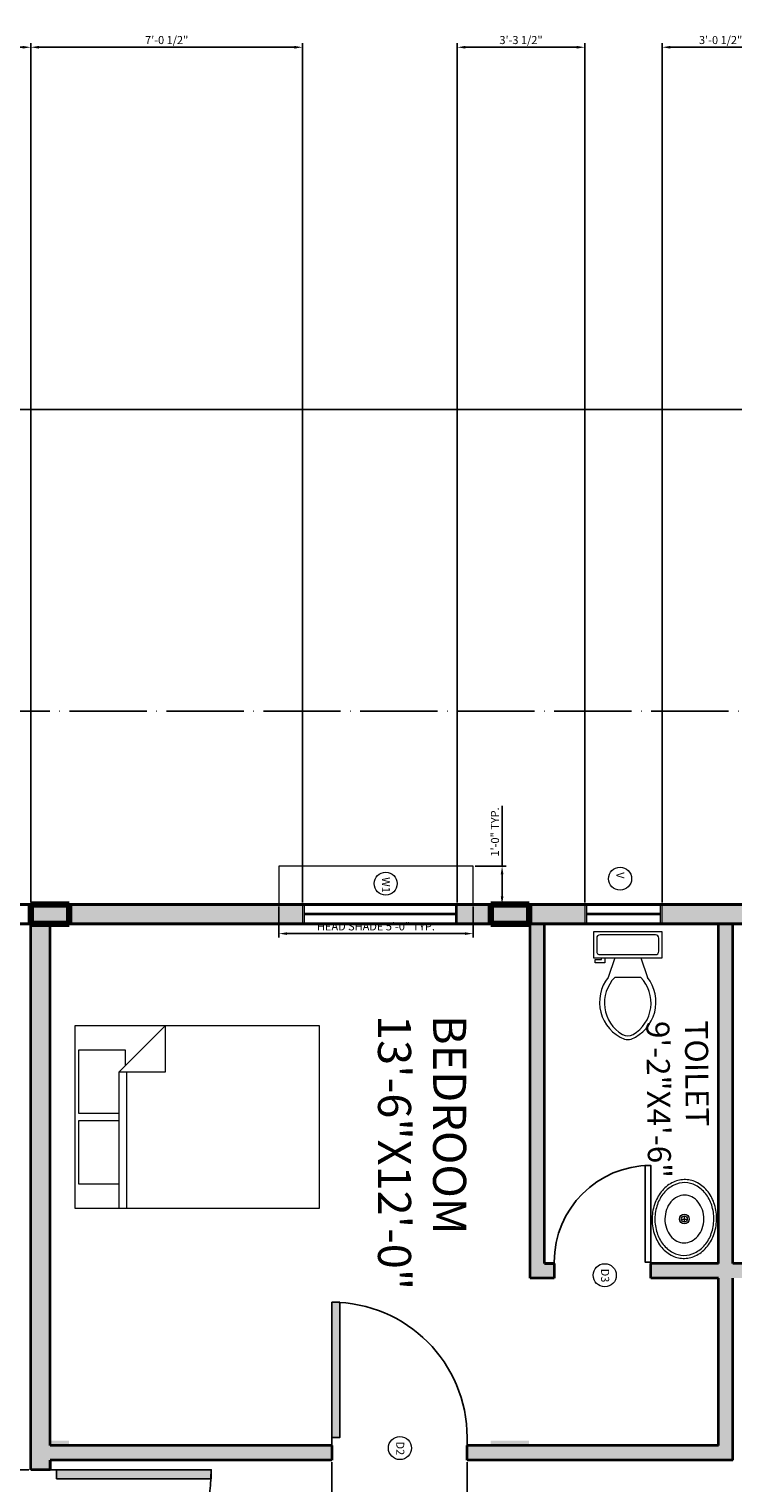
# Model space of a CAD drawing. Units: inches. Extents: x 7028582 to 7030319, y 63109697 to 63111305.
# Tile 17 of 18: x 7029748 to 7029966, y 63110853 to 63111305. Entities that reach past the tile are written whole.
import ezdxf

# ---------------------------------------------------------------- set-up
doc = ezdxf.new("R2010")
doc.units = ezdxf.units.IN
doc.linetypes.add('ACAD_ISO04W100', pattern=[30, 24, -3, 0, -3])
for name, color, linetype, lineweight in [('A-AREA-IDEN', 7, 'Continuous', 18), ('A-DOOR-IDEN', 20, 'Continuous', 13), ('A-FLOR-FIXT', 9, 'Continuous', 18), ('A-GLAZ-IDEN', 20, 'Continuous', 13), ('A-WALL-PATT', 8, 'Continuous', 13), ('C-ANNO-DIMS', 7, 'Continuous', 18), ('C-PROP', 1, 'ACAD_ISO04W100', 25), ('doors', 20, 'Continuous', 25), ('furniture', 9, 'Continuous', 18), ('PILLARS', 220, 'Continuous', 100), ('S-COLS-PATT', 220, 'Continuous', 100), ('walls', 6, 'Continuous', 35), ('WINDOW SHADOW', 9, 'Continuous', 13), ('windows', 5, 'Continuous', 18)]:
    doc.layers.add(name, color=color, linetype=linetype, lineweight=lineweight)
doc.styles.get("Standard").update_dxf_attribs({"font": 'arial.ttf'})
doc.dimstyles.new('ISO-25', dxfattribs={"dimtxt": 2.5, "dimasz": 2.5, "dimexe": 1.25, "dimexo": 0.625, "dimtad": 1, "dimlunit": 4, "dimtxsty": 'Standard', "dimcen": 2.5, "dimadec": 0, "dimazin": 0, "dimtfac": 1, "dimtmove": 0, "dimatfit": 3, "dimfxl": 1, "dimarcsym": 0})

# ---------------------------------------------------------------- blocks, each defined once
blk = doc.blocks.new('*U2')
for p, q in [((0, 0), (0, -5)), ((30, 0), (30, -5))]:
    blk.add_line(p, q)
blk.add_lwpolyline([(0, 0), (0, 30), (1.75, 30), (1.75, 0)], close=True)
blk.add_arc((0, 0), 30, 0, 90)
blk = doc.blocks.new('Toilet - top')
for p, q in [((9.5, -6), (9.5, -2)), ((-10, -8.5), (-8, -8.5)), ((-10, -9.5), (-10, -8.5)), ((-8, -8.5), (-8, -8)), ((-7, -8), (-7, -9.5)), ((-4, -8), (-6, -14)), ((4, -8), (6, -14)), ((-7, -9.5), (-10, -9.5)), ((4, -14), (-4, -14))]:
    blk.add_line(p, q)
blk.add_lwpolyline([(10.5, -8), (10.5, 0), (-10.5, 0), (-10.5, -8)], close=True)
for points in [[(-9.5, -2), (-9.5, -6)], [(8.5, -1), (-8.5, -1)], [(-8.5, -7), (8.5, -7)]]:
    blk.add_lwpolyline(points)
for centre, radius, start, end in [((-8.62, -1.88), 0.884, 81.8699, 188.1301), ((8.62, -1.88), 0.884, 351.8699, 98.1301), ((-8.62, -6.12), 0.884, 171.8699, 278.1301), ((8.62, -6.12), 0.884, 261.8699, 8.1301), ((3.52, -21.58), 12.17, 141.4691, 247.9714), ((4.2, -21.82), 11.33, 136.3677, 238.9468), ((-3.52, -21.58), 12.17, 292.0284, 38.5307), ((-4.2, -21.82), 11.33, 301.053, 43.6321), ((0, -27.88), 4, 245.7318, 294.2682), ((0, -29), 4, 254.8605, 285.1395)]:
    blk.add_arc(centre, radius, start, end)
blk = doc.blocks.new('Sink - Oval top')
for p, q in [((-1, 0), (1, 0)), ((0, 1), (0, -1))]:
    blk.add_line(p, q)
for points in [[(-12.23, 0.39, 0.117634), (-11.46, -3.36, 0.104469), (-8.88, -6.8, 0.090016), (-5.08, -9.07, 0.08192), (-0.32, -10.02, 0.08192), (4.49, -9.38, 0.090016), (8.42, -7.36, 0.104469), (11.22, -4.09, 0.117634), (12.23, -0.39, 0.117634), (11.46, 3.36, 0.104469), (8.88, 6.8, 0.090016), (5.08, 9.07, 0.08192), (0.32, 10.02, 0.08192), (-4.49, 9.38, 0.090016), (-8.42, 7.36, 0.104469), (-11.22, 4.09, 0.117634)], [(-11.29, 0.16, 0.118622), (-10.52, -3.25, 0.104678), (-8.07, -6.36, 0.089562), (-4.54, -8.37, 0.081185), (-0.13, -9.15, 0.081185), (4.3, -8.49, 0.089562), (7.89, -6.58, 0.104678), (10.42, -3.55, 0.118622), (11.29, -0.16, 0.118622), (10.52, 3.25, 0.104678), (8.07, 6.36, 0.089562), (4.54, 8.37, 0.081185), (0.13, 9.15, 0.081185), (-4.3, 8.49, 0.089562), (-7.89, 6.58, 0.104678), (-10.42, 3.55, 0.118622)], [(-7.42, 0.08, 0.118283), (-6.91, -2.17, 0.104607), (-5.29, -4.21, 0.089718), (-2.97, -5.53, 0.081436), (-0.07, -6.04, 0.081436), (2.84, -5.59, 0.089718), (5.2, -4.33, 0.104607), (6.86, -2.32, 0.118283), (7.42, -0.08, 0.118283), (6.91, 2.17, 0.104607), (5.29, 4.21, 0.089718), (2.97, 5.53, 0.081436), (0.07, 6.04, 0.081436), (-2.84, 5.59, 0.089718), (-5.2, 4.33, 0.104607), (-6.86, 2.32, 0.118283)]]:
    blk.add_lwpolyline(points, format="xyb", close=True)
for radius in [1.5, 1]:
    blk.add_circle((0, 0), radius)
blk = doc.blocks.new('Bed - Queen')
for p, q in [((0, -80.00003), (0, 0)), ((0, 0), (59.99999, 0)), ((59.99999, 0), (59.99999, -80.00003)), ((7.99999, -1.2), (28.79998, -1.2)), ((7.99999, -14.4), (7.99999, -1.2)), ((28.79998, -1.2), (28.79998, -14.4)), ((31.19999, -1.2), (51.99999, -1.2)), ((31.19999, -14.4), (31.19999, -1.2)), ((51.99999, -1.2), (51.99999, -16.4)), ((0, -14.4), (44.8, -14.4)), ((44.8, -16.8), (0, -16.8)), ((59.99999, -29.6), (44.8, -14.4)), ((44.8, -14.4), (44.8, -29.6)), ((51.99999, -16.4), (46.79936, -16.4)), ((44.8, -29.6), (59.99999, -29.6)), ((59.99999, -80.00003), (0, -80.00003))]:
    blk.add_line(p, q)
blk = doc.blocks.new('*D11')
at = {"layer": 'C-ANNO-DIMS', "color": 0, "lineweight": -2, "transparency": 16777216}
for p, q in [((7029174.71, 63111093.68), (7029174.71, 63111188.03)), ((7030233.21, 63111186.78), (7029177.21, 63111186.78)), ((7030235.71, 63111093.68), (7030235.71, 63111188.03))]:
    blk.add_line(p, q, dxfattribs=at)
at = {"layer": 'C-ANNO-DIMS', "color": 0, "lineweight": 100, "transparency": 16777216}
for points in [[(7029177.21, 63111187.2), (7029177.21, 63111186.36), (7029174.71, 63111186.78)], [(7030233.21, 63111187.2), (7030233.21, 63111186.36), (7030235.71, 63111186.78)]]:
    blk.add_solid(points, dxfattribs=at)
at = {"layer": 'Defpoints', "color": 0, "lineweight": 100, "transparency": 16777216}
for p in [(7029174.71, 63111186.78), (7029174.71, 63111093.06), (7030235.71, 63111093.06)]:
    blk.add_point(p, dxfattribs=at)
at = {"layer": 'C-ANNO-DIMS', "color": 0, "transparency": 16777216, "insert": (7029705.21, 63111193.53), "char_height": 12, "attachment_point": 5}
blk.add_mtext('88\'-5"', dxfattribs=at)
blk = doc.blocks.new('WIN-SASH-24')
for p, q in [((24.05, 6), (0, 6)), ((0.5, 6), (0.5, 0)), ((23.55, 0), (23.55, 6)), ((0, 0), (24.05, 0)), ((23.55, 3.2), (0.5, 3.2)), ((23.55, 2.8), (0.5, 2.8))]:
    blk.add_line(p, q)
blk = doc.blocks.new('WIN-SASH-48')
for p, q in [((48.05, 6), (0, 6)), ((0.5, 6), (0.5, 0)), ((47.55, 0), (47.55, 6)), ((47.55, 3.2), (0.5, 3.2)), ((47.55, 2.8), (0.5, 2.8)), ((0, 0), (48.05, 0))]:
    blk.add_line(p, q)
blk = doc.blocks.new('WINDOW-SHADE-HEAD-60')
for p, q in [((60.25, 11.9), (0, 11.9)), ((0, 11.9), (0, 0)), ((60.25, 0), (60.25, 11.9))]:
    blk.add_line(p, q)
blk = doc.blocks.new('TAG-D2-MT-R')
blk.add_circle((3.58, 3.58), 3.58)
at = {"insert": (4.93, 5.6), "char_height": 2.5, "attachment_point": 1, "rotation": 270}
blk.add_mtext_dynamic_manual_height_columns('D2', width=2.5021, gutter_width=12.5, heights=[0], dxfattribs=at)
blk = doc.blocks.new('TAG-D3-MT-R')
blk.add_circle((3.58, 3.58), 3.58)
at = {"insert": (4.93, 5.6), "char_height": 2.5, "attachment_point": 1, "rotation": 270}
blk.add_mtext_dynamic_manual_height_columns('D3', width=2.5021, gutter_width=12.5, heights=[0], dxfattribs=at)
blk = doc.blocks.new('TAG-V-MT-R')
blk.add_circle((3.58, 3.58), 3.58)
at = {"insert": (4.93, 5.6), "char_height": 2.5, "attachment_point": 1, "rotation": 270}
blk.add_mtext_dynamic_manual_height_columns('V', width=2.5021, gutter_width=12.5, heights=[0], dxfattribs=at)
blk = doc.blocks.new('TAG-W1-MT-R')
blk.add_circle((3.58, 3.58), 3.58)
at = {"insert": (4.93, 5.6), "char_height": 2.5, "attachment_point": 1, "rotation": 270}
blk.add_mtext_dynamic_manual_height_columns('W1', width=2.5021, gutter_width=12.5, heights=[0], dxfattribs=at)
blk = doc.blocks.new('*D91')
at = {"layer": 'C-ANNO-DIMS', "color": 0, "lineweight": -2, "transparency": 16777216}
for p, q in [((7029825.25, 63111032.43), (7029825.25, 63111022.77)), ((7029885.5, 63111032.43), (7029885.5, 63111022.77)), ((7029827.75, 63111024.02), (7029883, 63111024.02))]:
    blk.add_line(p, q, dxfattribs=at)
at = {"layer": 'C-ANNO-DIMS', "color": 0, "lineweight": 100, "transparency": 16777216}
for points in [[(7029827.75, 63111024.44), (7029827.75, 63111023.6), (7029825.25, 63111024.02)], [(7029883, 63111024.44), (7029883, 63111023.6), (7029885.5, 63111024.02)]]:
    blk.add_solid(points, dxfattribs=at)
at = {"layer": 'Defpoints', "color": 0, "lineweight": 100, "transparency": 16777216}
for p in [(7029825.25, 63111033.06), (7029885.5, 63111033.06), (7029885.5, 63111024.02)]:
    blk.add_point(p, dxfattribs=at)
at = {"layer": 'C-ANNO-DIMS', "color": 0, "transparency": 16777216, "insert": (7029855.37, 63111025.94), "char_height": 2.5, "attachment_point": 5}
blk.add_mtext('HEAD SHADE 5\'-0" TYP.', dxfattribs=at)
blk = doc.blocks.new('*D92')
at = {"layer": 'C-ANNO-DIMS', "color": 0, "lineweight": -2, "transparency": 16777216}
for p, q in [((7029894.53, 63111044.96), (7029894.53, 63111063.71)), ((7029886.12, 63111044.96), (7029895.78, 63111044.96)), ((7029894.53, 63111035.56), (7029894.53, 63111042.46)), ((7029886.12, 63111033.06), (7029895.78, 63111033.06))]:
    blk.add_line(p, q, dxfattribs=at)
at = {"layer": 'C-ANNO-DIMS', "color": 0, "lineweight": 100, "transparency": 16777216}
for points in [[(7029894.12, 63111042.46), (7029894.95, 63111042.46), (7029894.53, 63111044.96)], [(7029894.12, 63111035.56), (7029894.95, 63111035.56), (7029894.53, 63111033.06)]]:
    blk.add_solid(points, dxfattribs=at)
at = {"layer": 'Defpoints', "color": 0, "lineweight": 100, "transparency": 16777216}
for p in [(7029885.5, 63111044.96), (7029894.53, 63111044.96), (7029885.5, 63111033.06)]:
    blk.add_point(p, dxfattribs=at)
at = {"layer": 'C-ANNO-DIMS', "color": 0, "transparency": 16777216, "insert": (7029892.63, 63111055.58), "char_height": 2.5, "attachment_point": 5, "rotation": 90}
blk.add_mtext('1\'-0" TYP.', dxfattribs=at)
blk = doc.blocks.new('*D102')
at = {"layer": 'C-ANNO-DIMS', "color": 0, "lineweight": -2, "transparency": 16777216}
for p, q in [((7029662.21, 63111033.68), (7029662.21, 63111300.44)), ((7029664.71, 63111299.19), (7029745.71, 63111299.19)), ((7029748.21, 63111033.68), (7029748.21, 63111300.44))]:
    blk.add_line(p, q, dxfattribs=at)
at = {"layer": 'C-ANNO-DIMS', "color": 0, "lineweight": 100, "transparency": 16777216}
for points in [[(7029664.71, 63111299.61), (7029664.71, 63111298.77), (7029662.21, 63111299.19)], [(7029745.71, 63111299.61), (7029745.71, 63111298.77), (7029748.21, 63111299.19)]]:
    blk.add_solid(points, dxfattribs=at)
at = {"layer": 'Defpoints', "color": 0, "lineweight": 100, "transparency": 16777216}
for p in [(7029748.21, 63111299.19), (7029662.21, 63111033.06), (7029748.21, 63111033.06)]:
    blk.add_point(p, dxfattribs=at)
at = {"layer": 'C-ANNO-DIMS', "color": 0, "transparency": 16777216, "insert": (7029705.21, 63111301.07), "char_height": 2.5, "attachment_point": 5}
blk.add_mtext('7\'-2"', dxfattribs=at)
blk = doc.blocks.new('*D104')
at = {"layer": 'C-ANNO-DIMS', "color": 0, "lineweight": -2, "transparency": 16777216}
for p, q in [((7029747.58, 63110857.56), (7028586.23, 63110857.56)), ((7028587.48, 63110812.06), (7028587.48, 63110855.06)), ((7029747.58, 63110809.56), (7028586.23, 63110809.56))]:
    blk.add_line(p, q, dxfattribs=at)
at = {"layer": 'C-ANNO-DIMS', "color": 0, "lineweight": 100, "transparency": 16777216}
for points in [[(7028587.06, 63110855.06), (7028587.89, 63110855.06), (7028587.48, 63110857.56)], [(7028587.06, 63110812.06), (7028587.89, 63110812.06), (7028587.48, 63110809.56)]]:
    blk.add_solid(points, dxfattribs=at)
at = {"layer": 'Defpoints', "color": 0, "lineweight": 100, "transparency": 16777216}
for p in [(7028587.48, 63110857.56), (7029748.21, 63110857.56), (7029748.21, 63110809.56)]:
    blk.add_point(p, dxfattribs=at)
at = {"layer": 'C-ANNO-DIMS', "color": 0, "transparency": 16777216, "insert": (7028585.57, 63110833.56), "char_height": 2.5, "attachment_point": 5, "rotation": 90}
blk.add_mtext('4\'-0"', dxfattribs=at)
blk = doc.blocks.new('*D105')
at = {"layer": 'C-ANNO-DIMS', "color": 0, "lineweight": -2, "transparency": 16777216}
for p, q in [((7029841.68, 63110859.93), (7029841.68, 63109697.14)), ((7029883.68, 63110859.93), (7029883.68, 63109697.14)), ((7029844.18, 63109698.39), (7029881.18, 63109698.39))]:
    blk.add_line(p, q, dxfattribs=at)
at = {"layer": 'C-ANNO-DIMS', "color": 0, "lineweight": 100, "transparency": 16777216}
for points in [[(7029844.18, 63109698.8), (7029844.18, 63109697.97), (7029841.68, 63109698.39)], [(7029881.18, 63109698.8), (7029881.18, 63109697.97), (7029883.68, 63109698.39)]]:
    blk.add_solid(points, dxfattribs=at)
at = {"layer": 'Defpoints', "color": 0, "lineweight": 100, "transparency": 16777216}
for p in [(7029841.68, 63110860.56), (7029883.68, 63110860.56), (7029883.68, 63109698.39)]:
    blk.add_point(p, dxfattribs=at)
at = {"layer": 'C-ANNO-DIMS', "color": 0, "transparency": 16777216, "insert": (7029862.68, 63109700.29), "char_height": 2.5, "attachment_point": 5}
blk.add_mtext('3\'-6"', dxfattribs=at)
blk = doc.blocks.new('*D112')
at = {"layer": 'C-ANNO-DIMS', "color": 0, "lineweight": -2, "transparency": 16777216}
for p, q in [((7029747.58, 63111033.06), (7028586.23, 63111033.06)), ((7028587.48, 63111030.56), (7028587.48, 63110548.06)), ((7029747.58, 63110545.56), (7028586.23, 63110545.56))]:
    blk.add_line(p, q, dxfattribs=at)
at = {"layer": 'C-ANNO-DIMS', "color": 0, "lineweight": 100, "transparency": 16777216}
for points in [[(7028587.06, 63111030.56), (7028587.89, 63111030.56), (7028587.48, 63111033.06)], [(7028587.06, 63110548.06), (7028587.89, 63110548.06), (7028587.48, 63110545.56)]]:
    blk.add_solid(points, dxfattribs=at)
at = {"layer": 'Defpoints', "color": 0, "lineweight": 100, "transparency": 16777216}
for p in [(7029748.21, 63111033.06), (7028587.48, 63110545.56), (7029748.21, 63110545.56)]:
    blk.add_point(p, dxfattribs=at)
at = {"layer": 'C-ANNO-DIMS', "color": 0, "transparency": 16777216, "insert": (7028585.56, 63110789.31), "char_height": 2.5, "attachment_point": 5, "rotation": 90}
blk.add_mtext('40\'-7 1/2"', dxfattribs=at)
blk = doc.blocks.new('*D113')
at = {"layer": 'C-ANNO-DIMS', "color": 0, "lineweight": -2, "transparency": 16777216}
for p, q in [((7029748.21, 63111033.68), (7029748.21, 63111300.44)), ((7029750.71, 63111299.19), (7029830.07, 63111299.19)), ((7029832.57, 63111033.68), (7029832.57, 63111300.44))]:
    blk.add_line(p, q, dxfattribs=at)
at = {"layer": 'C-ANNO-DIMS', "color": 0, "lineweight": 100, "transparency": 16777216}
for points in [[(7029750.71, 63111299.61), (7029750.71, 63111298.77), (7029748.21, 63111299.19)], [(7029830.07, 63111299.61), (7029830.07, 63111298.77), (7029832.57, 63111299.19)]]:
    blk.add_solid(points, dxfattribs=at)
at = {"layer": 'Defpoints', "color": 0, "lineweight": 100, "transparency": 16777216}
for p in [(7029832.57, 63111299.19), (7029748.21, 63111033.06), (7029832.57, 63111033.06)]:
    blk.add_point(p, dxfattribs=at)
at = {"layer": 'C-ANNO-DIMS', "color": 0, "transparency": 16777216, "insert": (7029790.39, 63111301.11), "char_height": 2.5, "attachment_point": 5}
blk.add_mtext('7\'-0 1/2"', dxfattribs=at)
blk = doc.blocks.new('*D114')
at = {"layer": 'C-ANNO-DIMS', "color": 0, "lineweight": -2, "transparency": 16777216}
for p, q in [((7029880.62, 63111033.68), (7029880.62, 63111300.44)), ((7029883.12, 63111299.19), (7029917.71, 63111299.19)), ((7029920.21, 63111033.68), (7029920.21, 63111300.44))]:
    blk.add_line(p, q, dxfattribs=at)
at = {"layer": 'C-ANNO-DIMS', "color": 0, "lineweight": 100, "transparency": 16777216}
for points in [[(7029883.12, 63111299.61), (7029883.12, 63111298.77), (7029880.62, 63111299.19)], [(7029917.71, 63111299.61), (7029917.71, 63111298.77), (7029920.21, 63111299.19)]]:
    blk.add_solid(points, dxfattribs=at)
at = {"layer": 'Defpoints', "color": 0, "lineweight": 100, "transparency": 16777216}
for p in [(7029920.21, 63111299.19), (7029880.62, 63111033.06), (7029920.21, 63111033.06)]:
    blk.add_point(p, dxfattribs=at)
at = {"layer": 'C-ANNO-DIMS', "color": 0, "transparency": 16777216, "insert": (7029900.41, 63111301.11), "char_height": 2.5, "attachment_point": 5}
blk.add_mtext('3\'-3 1/2"', dxfattribs=at)
blk = doc.blocks.new('*D115')
at = {"layer": 'C-ANNO-DIMS', "color": 0, "lineweight": -2, "transparency": 16777216}
for p, q in [((7029944.26, 63111033.68), (7029944.26, 63111300.44)), ((7029946.76, 63111299.19), (7029978.03, 63111299.19)), ((7029980.53, 63111033.68), (7029980.53, 63111300.44))]:
    blk.add_line(p, q, dxfattribs=at)
at = {"layer": 'C-ANNO-DIMS', "color": 0, "lineweight": 100, "transparency": 16777216}
for points in [[(7029946.76, 63111299.61), (7029946.76, 63111298.77), (7029944.26, 63111299.19)], [(7029978.03, 63111299.61), (7029978.03, 63111298.77), (7029980.53, 63111299.19)]]:
    blk.add_solid(points, dxfattribs=at)
at = {"layer": 'Defpoints', "color": 0, "lineweight": 100, "transparency": 16777216}
for p in [(7029980.53, 63111299.19), (7029944.26, 63111033.06), (7029980.53, 63111033.06)]:
    blk.add_point(p, dxfattribs=at)
at = {"layer": 'C-ANNO-DIMS', "color": 0, "transparency": 16777216, "insert": (7029962.39, 63111301.11), "char_height": 2.5, "attachment_point": 5}
blk.add_mtext('3\'-0 1/2"', dxfattribs=at)

msp = doc.modelspace()

# ---------------------------------------------------------------- hatches: boundary and pattern name
at = {"layer": 'A-WALL-PATT'}
h = msp.add_hatch(color=256, dxfattribs=at)
h.dxf.hatch_style = 1
h.paths.add_polyline_path([(7029832.57, 63111033.057), (7029748.205, 63111033.057), (7029748.205, 63111027.057), (7029832.57, 63111027.057)])
h = msp.add_hatch(color=256, dxfattribs=at)
h.dxf.hatch_style = 1
h.paths.add_polyline_path([(7029920.21, 63111033.057), (7029880.618, 63111033.057), (7029880.618, 63111027.057), (7029920.21, 63111027.057)])
h = msp.add_hatch(color=256, dxfattribs=at)
h.dxf.hatch_style = 1
h.paths.add_polyline_path([(7029980.53, 63111033.057), (7029944.258, 63111033.057), (7029944.258, 63111027.057), (7029980.53, 63111027.057)])
h = msp.add_hatch(color=256, dxfattribs=at)
h.dxf.hatch_style = 1
h.paths.add_polyline_path([(7029754.205, 63110857.557), (7029756.205, 63110857.557), (7029804.205, 63110857.557), (7029804.205, 63110854.757), (7029756.205, 63110854.757), (7029756.205, 63110857.557), (7029748.205, 63110857.557), (7029748.205, 63111027.057), (7029754.205, 63111027.057), (7029754.205, 63110865.057), (7029841.685, 63110865.057), (7029841.685, 63110867.557), (7029841.685, 63110909.557), (7029844.135, 63110909.557), (7029844.135, 63110867.557), (7029841.685, 63110867.557), (7029841.685, 63110860.557), (7029754.205, 63110860.557)])
h = msp.add_hatch(color=256, dxfattribs=at)
h.dxf.hatch_style = 1
h.paths.add_polyline_path([(7030025.705, 63111027.057), (7030021.205, 63111027.057), (7030021.205, 63110954.557), (7030025.705, 63110954.557)], flags=0)
h.paths.add_polyline_path([(7030025.705, 63110924.557), (7030021.205, 63110924.557), (7030021.205, 63110921.557), (7029966.205, 63110921.557), (7029966.205, 63111027.057), (7029961.705, 63111027.057), (7029961.705, 63110921.557), (7029940.705, 63110921.557), (7029940.705, 63110917.057), (7029961.705, 63110917.057), (7029961.705, 63110865.057), (7029883.685, 63110865.057), (7029883.685, 63110860.557), (7029966.205, 63110860.557), (7029966.205, 63110917.057), (7030021.205, 63110917.057), (7030021.205, 63110910.057), (7030025.705, 63110910.057)])
h = msp.add_hatch(color=256, dxfattribs=at)
h.dxf.hatch_style = 1
h.paths.add_polyline_path([(7029907.705, 63111027.057), (7029903.205, 63111027.057), (7029903.205, 63110917.057), (7029910.705, 63110917.057), (7029910.705, 63110921.557), (7029907.705, 63110921.557)], flags=17)
at = {"layer": 'S-COLS-PATT'}
h = msp.add_hatch(color=256, dxfattribs=at)
h.dxf.hatch_style = 1
h.paths.add_polyline_path([(7029760.108, 63111033.057), (7029748.205, 63111033.057), (7029748.205, 63111027.057), (7029760.108, 63111027.057)])
h = msp.add_hatch(color=256, dxfattribs=at)
h.dxf.hatch_style = 1
h.paths.add_polyline_path([(7029902.915, 63111033.057), (7029891, 63111033.057), (7029891, 63111027.057), (7029902.915, 63111027.057)])
h = msp.add_hatch(color=256, dxfattribs=at)
h.dxf.hatch_style = 1
h.paths.add_polyline_path([(7029760.108, 63110866.557), (7029748.205, 63110866.557), (7029748.205, 63110860.557), (7029760.108, 63110860.557)])
h = msp.add_hatch(color=256, dxfattribs=at)
h.dxf.hatch_style = 1
h.paths.add_polyline_path([(7029902.915, 63110866.557), (7029891, 63110866.557), (7029891, 63110860.557), (7029902.915, 63110860.557)])

# ---------------------------------------------------------------- linework, layer by layer
at = {"layer": 'C-PROP'}
msp.add_line((7030235.705, 63111093.057), (7029174.705, 63111093.057), dxfattribs=at)
at = {"layer": 'PILLARS'}
for p, q in [((7029760.108, 63111033.057), (7029748.193, 63111033.057)), ((7029748.193, 63111033.057), (7029748.193, 63111027.057)), ((7029760.108, 63111027.057), (7029760.108, 63111033.057)), ((7029902.915, 63111033.057), (7029891, 63111033.057)), ((7029891, 63111033.057), (7029891, 63111027.057)), ((7029902.915, 63111027.057), (7029902.915, 63111033.057)), ((7029748.193, 63111027.057), (7029760.108, 63111027.057)), ((7029891, 63111027.057), (7029902.915, 63111027.057))]:
    msp.add_line(p, q, dxfattribs=at)
at = {"layer": 'walls'}
for p, q in [((7030175.705, 63111033.057), (7029234.705, 63111033.057)), ((7029234.705, 63111033.057), (7030175.705, 63111033.057)), ((7029748.205, 63110857.557), (7029748.205, 63111033.057)), ((7030169.705, 63111027.057), (7029240.705, 63111027.057)), ((7029240.705, 63111027.057), (7030169.705, 63111027.057)), ((7029754.205, 63110865.057), (7029754.205, 63111027.057)), ((7029903.205, 63110917.057), (7029903.205, 63111027.057)), ((7029907.705, 63110921.557), (7029907.705, 63111027.057)), ((7029961.705, 63110921.557), (7029961.705, 63111027.057)), ((7029966.205, 63110921.557), (7029966.205, 63111027.057)), ((7029907.705, 63110921.557), (7029910.705, 63110921.557)), ((7029910.705, 63110921.557), (7029907.705, 63110921.557)), ((7029910.705, 63110921.557), (7029910.705, 63110917.057)), ((7029940.705, 63110917.057), (7029940.705, 63110921.557)), ((7029961.705, 63110921.557), (7029940.705, 63110921.557)), ((7030021.205, 63110921.557), (7029966.205, 63110921.557)), ((7029910.705, 63110917.057), (7029903.205, 63110917.057)), ((7029961.705, 63110917.057), (7029940.705, 63110917.057)), ((7029961.705, 63110865.057), (7029961.705, 63110917.057)), ((7029966.205, 63110860.557), (7029966.205, 63110917.057)), ((7029841.685, 63110865.057), (7029754.205, 63110865.057)), ((7029841.685, 63110865.057), (7029841.685, 63110860.557)), ((7029883.685, 63110860.557), (7029883.685, 63110865.057)), ((7029961.705, 63110865.057), (7029883.685, 63110865.057)), ((7029841.685, 63110860.557), (7029754.205, 63110860.557)), ((7029754.205, 63110860.557), (7029754.205, 63110857.557)), ((7029754.205, 63110857.557), (7029754.205, 63110860.557)), ((7029966.205, 63110860.557), (7029883.685, 63110860.557)), ((7029754.205, 63110857.557), (7029748.205, 63110857.557))]:
    msp.add_line(p, q, dxfattribs=at)
at = {"layer": 'windows'}
for p, q in [((7029832.57, 63111033.057), (7029832.57, 63111027.057)), ((7029880.618, 63111027.057), (7029880.618, 63111033.057)), ((7029920.21, 63111033.057), (7029920.21, 63111027.057)), ((7029944.258, 63111027.057), (7029944.258, 63111033.057))]:
    msp.add_line(p, q, dxfattribs=at)

# ---------------------------------------------------------------- block references
at = {"layer": 'A-DOOR-IDEN'}
for name, p in [('TAG-D3-MT-R', (7029922.838, 63110914.381)), ('TAG-D2-MT-R', (7029859.234, 63110860.722))]:
    msp.add_blockref(name, p, dxfattribs=at)
at = {"layer": 'A-FLOR-FIXT', "xscale": 1.013555723357934, "yscale": 1.013555723357934, "zscale": 1.013555723357934}
msp.add_blockref('Toilet - top', (7029933.551, 63111024.605), dxfattribs=at)
at = {"layer": 'A-FLOR-FIXT', "rotation": 90}
msp.add_blockref('Sink - Oval top', (7029951.122, 63110935.416), dxfattribs=at)
at = {"layer": 'A-GLAZ-IDEN'}
for name, p in [('TAG-W1-MT-R', (7029854.806, 63111035.953)), ('TAG-V-MT-R', (7029927.584, 63111037.489))]:
    msp.add_blockref(name, p, dxfattribs=at)
at = {"layer": 'doors', "xscale": -1}
msp.add_blockref('*U2', (7029940.705, 63110922.057), dxfattribs=at)
at = {"layer": 'doors', "xscale": 1.399999999999999, "yscale": 1.399999999999999, "zscale": 1.399999999999999}
msp.add_blockref('*U2', (7029841.685, 63110867.557), dxfattribs=at)
at = {"layer": 'doors', "xscale": 1.599999999999999, "yscale": 1.599999999999999, "zscale": 1.599999999999999, "rotation": 270}
msp.add_blockref('*U2', (7029756.205, 63110857.557), dxfattribs=at)
at = {"layer": 'furniture', "xscale": 0.9464141645025947, "yscale": 0.9464141645025947, "zscale": 0.9464141645025947, "rotation": 89.99999999999999}
msp.add_blockref('Bed - Queen', (7029761.974, 63110938.688), dxfattribs=at)
at = {"layer": 'WINDOW SHADOW'}
msp.add_blockref('WINDOW-SHADE-HEAD-60', (7029825.251, 63111033.057), dxfattribs=at)
at = {"layer": 'windows'}
for name, p in [('WIN-SASH-48', (7029832.57, 63111027.057)), ('WIN-SASH-24', (7029920.21, 63111027.057))]:
    msp.add_blockref(name, p, dxfattribs=at)

# ---------------------------------------------------------------- texts
at = {"layer": 'A-AREA-IDEN', "attachment_point": 1}
for s, width, gutter_width, insert, char_height, rotation in [('BEDROOM\\P13\'-6"X12\'-0"', 82.04322, 51.315, (7029883.378, 63110998.737), 10.26307, 270), ('TOILET\\P9\'-2"X4\'-6"', 42.97461, 35.821, (7029958.409, 63110997.065), 7.16426, 270.6464)]:
    msp.add_mtext_dynamic_manual_height_columns(s, width=width, gutter_width=gutter_width, heights=[0], dxfattribs=dict(at, insert=insert, char_height=char_height, rotation=rotation))

# ---------------------------------------------------------------- dimensions: what is measured, and where the dimension line sits
at = {"layer": 'C-ANNO-DIMS'}
for base, p1, p2, override, picture, middle in [((7029832.57, 63111299.19), (7029748.205, 63111033.057), (7029832.57, 63111033.057), {"dimdec": 1, "dimlfac": 1, "dimrnd": 0, "dimzin": 1, "dimdsep": 46, "dimlunit": 4, "dimfrac": 2}, '*D113', (7029790.387, 63111301.107)), ((7029920.21, 63111299.19), (7029880.618, 63111033.057), (7029920.21, 63111033.057), {"dimdec": 1, "dimlfac": 1, "dimrnd": 0, "dimzin": 1, "dimdsep": 46, "dimlunit": 4, "dimfrac": 2}, '*D114', (7029900.414, 63111301.108)), ((7029980.53, 63111299.19), (7029944.258, 63111033.057), (7029980.53, 63111033.057), {"dimdec": 1, "dimlfac": 1, "dimrnd": 0, "dimzin": 1, "dimdsep": 46, "dimlunit": 4, "dimfrac": 2}, '*D115', (7029962.394, 63111301.108)), ((7029748.205, 63111299.19), (7029662.205, 63111033.057), (7029748.205, 63111033.057), {"dimdec": 1, "dimlfac": 1, "dimrnd": 0, "dimzin": 1, "dimdsep": 46, "dimlunit": 4, "dimfrac": 2}, '*D102', (7029705.205, 63111301.07)), ((7029174.705, 63111186.781), (7030235.705, 63111093.057), (7029174.705, 63111093.057), {"dimtxt": 12, "dimclrd": 0, "dimclre": 0, "dimclrt": 0}, '*D11', (7029705.205, 63111193.533)), ((7029883.685, 63109698.385), (7029841.685, 63110860.557), (7029883.685, 63110860.557), {"dimdec": 1, "dimlfac": 1, "dimrnd": 0, "dimzin": 1, "dimdsep": 46, "dimlunit": 4, "dimfrac": 2}, '*D105', (7029862.685, 63109700.288))]:
    dim = msp.add_linear_dim(base=base, p1=p1, p2=p2, dimstyle='ISO-25', override=override, dxfattribs=at)
    dim.commit()
    dim.dimension.update_dxf_attribs({"geometry": picture, "text_midpoint": middle})
dim = msp.add_linear_dim(base=(7029894.535, 63111044.957), p1=(7029885.498, 63111033.057), p2=(7029885.498, 63111044.957), angle=90, text='<> TYP.', dimstyle='ISO-25', override={"dimdec": 1, "dimlfac": 1, "dimrnd": 0, "dimzin": 1, "dimdsep": 46, "dimlunit": 4, "dimfrac": 2}, dxfattribs=at)
dim.commit()
dim.dimension.update_dxf_attribs({"geometry": '*D92', "text_midpoint": (7029892.633, 63111055.584)})
for base, p1, p2, picture, middle in [((7028587.475, 63110545.557), (7029748.205, 63111033.057), (7029748.205, 63110545.557), '*D112', (7028585.558, 63110789.307)), ((7028587.475, 63110857.557), (7029748.205, 63110809.557), (7029748.205, 63110857.557), '*D104', (7028585.574, 63110833.557))]:
    dim = msp.add_linear_dim(base=base, p1=p1, p2=p2, angle=90, dimstyle='ISO-25', override={"dimdec": 1, "dimlfac": 1, "dimrnd": 0, "dimzin": 1, "dimdsep": 46, "dimlunit": 4, "dimfrac": 2}, dxfattribs=at)
    dim.commit()
    dim.dimension.update_dxf_attribs({"geometry": picture, "text_midpoint": middle})
dim = msp.add_linear_dim(base=(7029885.498, 63111024.02), p1=(7029825.251, 63111033.057), p2=(7029885.498, 63111033.057), text='HEAD SHADE <> TYP.', dimstyle='ISO-25', override={"dimdec": 1, "dimlfac": 1, "dimrnd": 0, "dimzin": 1, "dimdsep": 46, "dimlunit": 4, "dimfrac": 2}, dxfattribs=at)
dim.commit()
dim.dimension.update_dxf_attribs({"geometry": '*D91', "text_midpoint": (7029855.374, 63111025.937)})

doc.saveas('drawing.dxf')
